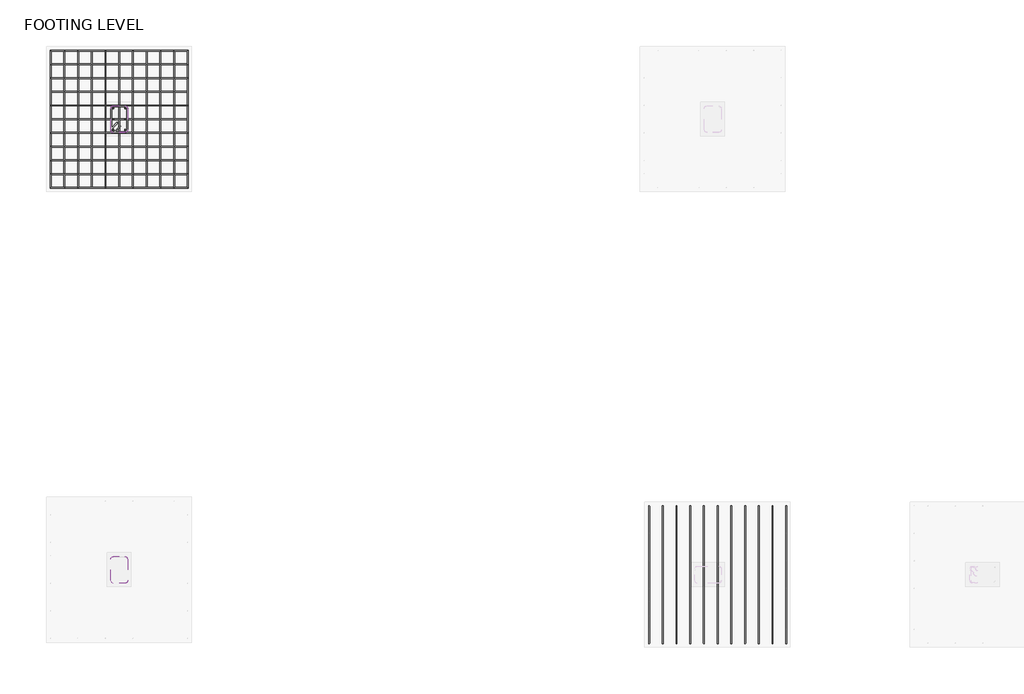
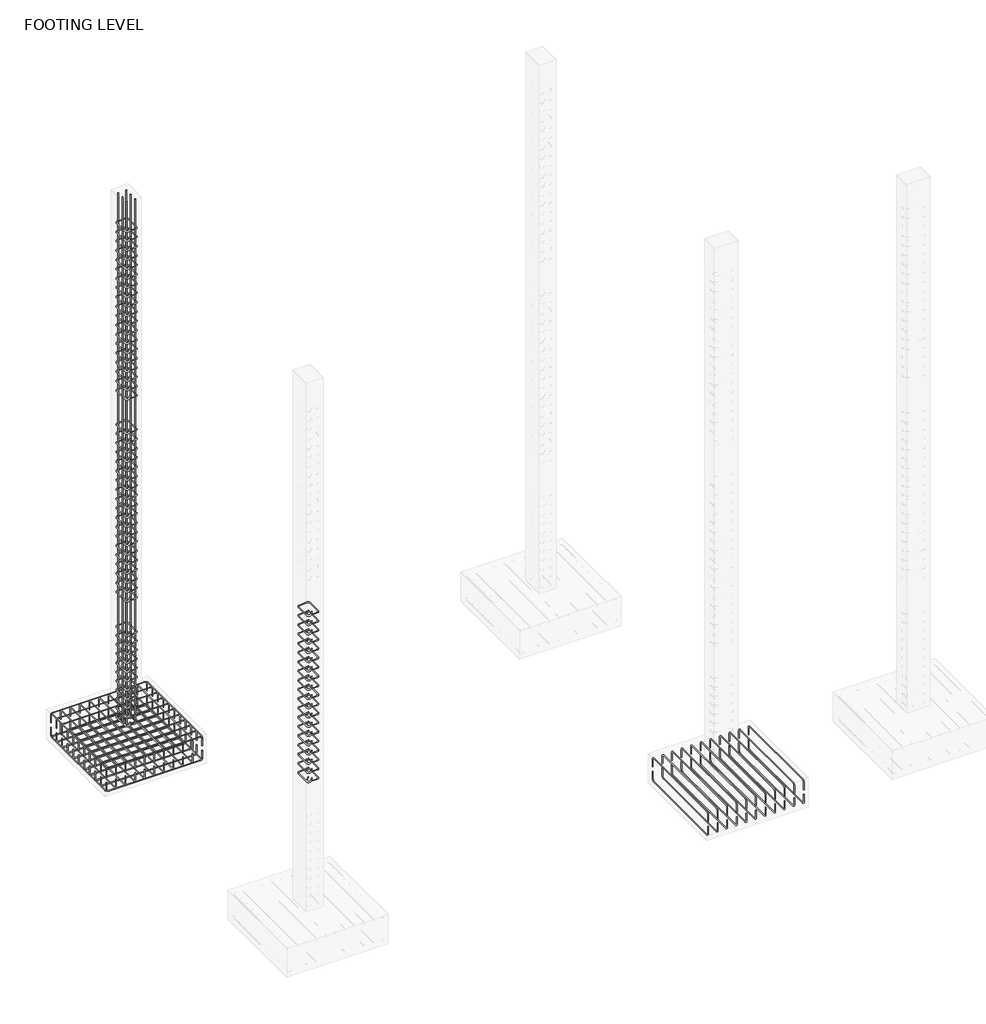
# One storey, part 7 of 9: 16 reinforcing bars.
"""IFC4 building model written with IfcOpenShell, lengths in millimetres."""

from ifc_helpers import new_model, si_unit, point, frame, origin, place, context, project, spatial, polyline, circle_curve, trimmed, segment, composite_curve, source, transform, mapped, element, save
from ifc_brep_helpers import swept_disk

model = new_model("IFC4")

# Units and contexts
model_context = context("Model", 3, world=origin())
ifc_project = project(units=[si_unit("LENGTHUNIT", "METRE", prefix="MILLI")], contexts=[model_context])

# Site, building, storey
site = spatial("IfcSite", under=ifc_project)
building = spatial("IfcBuilding", under=site)
storey = spatial("IfcBuildingStorey", under=building, Name="FOOTING LEVEL", Elevation=-1981.2)

# Reinforcing bars
placement = place(None, origin())
reinforcing_bar_shape = source(origin(), model_context, "Body", "SolidModel", [
    swept_disk(composite_curve([segment(polyline([(-5369.1458659, 8895.7158402, -2171.7), (-5369.1458659, 8895.7158402, -2057.4)]), True, "CONTINUOUS"), segment(trimmed(circle_curve(frame((-5369.1458659, 8862.3783402, -2057.4), z_axis=(1.0, 0.0, 0.0), x_axis=(0.0, 33.337499999999636, 0.0)), 33.3375), [point((-5369.1458659, 8895.7158402, -2057.4))], [point((-5369.1458659, 8862.3783402, -2024.0625))], True, "CARTESIAN"), True, "CONTINUOUS"), segment(polyline([(-5369.1458659, 8862.3783402, -2024.0625), (-5369.1458659, 7490.7783402, -2024.0625)]), True, "CONTINUOUS"), segment(trimmed(circle_curve(frame((-5369.1458659, 7490.7783402, -2057.4), z_axis=(1.0, 0.0, 0.0), x_axis=(0.0, 0.0, 33.33750000000009)), 33.3375), [point((-5369.1458659, 7490.7783402, -2024.0625))], [point((-5369.1458659, 7457.4408402, -2057.4))], True, "CARTESIAN"), True, "CONTINUOUS"), segment(polyline([(-5369.1458659, 7457.4408402, -2057.4), (-5369.1458659, 7457.4408402, -2171.7)]), True, "CONTINUOUS")], self_intersect=False), 4.7625),
])
element("IfcReinforcingBar", 1, at=placement, inside=storey, context=model_context, shape_type="MappedRepresentation", body=[
    mapped(reinforcing_bar_shape, transform((0.0, 0.0, 0.0), x_axis=(1.0, 0.0, 0.0), y_axis=(0.0, 1.0, 0.0), z_axis=(0.0, 0.0, 1.0))),
    mapped(reinforcing_bar_shape, transform((-143.8275, 0.0, 0.0), x_axis=(1.0, 0.0, 0.0), y_axis=(0.0, 1.0, 0.0), z_axis=(0.0, 0.0, 1.0))),
    mapped(reinforcing_bar_shape, transform((-287.655, 0.0, 0.0), x_axis=(1.0, 0.0, 0.0), y_axis=(0.0, 1.0, 0.0), z_axis=(0.0, 0.0, 1.0))),
    mapped(reinforcing_bar_shape, transform((-431.4825, 0.0, 0.0), x_axis=(1.0, 0.0, 0.0), y_axis=(0.0, 1.0, 0.0), z_axis=(0.0, 0.0, 1.0))),
    mapped(reinforcing_bar_shape, transform((-575.31, 0.0, 0.0), x_axis=(1.0, 0.0, 0.0), y_axis=(0.0, 1.0, 0.0), z_axis=(0.0, 0.0, 1.0))),
    mapped(reinforcing_bar_shape, transform((-719.1375, 0.0, 0.0), x_axis=(1.0, 0.0, 0.0), y_axis=(0.0, 1.0, 0.0), z_axis=(0.0, 0.0, 1.0))),
    mapped(reinforcing_bar_shape, transform((-862.965, 0.0, 0.0), x_axis=(1.0, 0.0, 0.0), y_axis=(0.0, 1.0, 0.0), z_axis=(0.0, 0.0, 1.0))),
    mapped(reinforcing_bar_shape, transform((-1006.7925, 0.0, 0.0), x_axis=(1.0, 0.0, 0.0), y_axis=(0.0, 1.0, 0.0), z_axis=(0.0, 0.0, 1.0))),
    mapped(reinforcing_bar_shape, transform((-1150.62, 0.0, 0.0), x_axis=(1.0, 0.0, 0.0), y_axis=(0.0, 1.0, 0.0), z_axis=(0.0, 0.0, 1.0))),
    mapped(reinforcing_bar_shape, transform((-1294.4475, 0.0, 0.0), x_axis=(1.0, 0.0, 0.0), y_axis=(0.0, 1.0, 0.0), z_axis=(0.0, 0.0, 1.0))),
    mapped(reinforcing_bar_shape, transform((-1438.275, 0.0, 0.0), x_axis=(1.0, 0.0, 0.0), y_axis=(0.0, 1.0, 0.0), z_axis=(0.0, 0.0, 1.0))),
])
reinforcing_bar_2_shape = source(origin(), model_context, "Body", "SolidModel", [
    swept_disk(composite_curve([segment(polyline([(-5369.1458659, 7457.4408402, -2247.9), (-5369.1458659, 7457.4408402, -2362.2)]), True, "CONTINUOUS"), segment(trimmed(circle_curve(frame((-5369.1458659, 7490.7783402, -2362.2), z_axis=(1.0, 0.0, 0.0), x_axis=(0.0, -33.337499999999636, 0.0)), 33.3375), [point((-5369.1458659, 7457.4408402, -2362.2))], [point((-5369.1458659, 7490.7783402, -2395.5375))], True, "CARTESIAN"), True, "CONTINUOUS"), segment(polyline([(-5369.1458659, 7490.7783402, -2395.5375), (-5369.1458659, 8862.3783402, -2395.5375)]), True, "CONTINUOUS"), segment(trimmed(circle_curve(frame((-5369.1458659, 8862.3783402, -2362.2), z_axis=(1.0, 0.0, 0.0), x_axis=(0.0, 0.0, -33.33750000000009)), 33.3375), [point((-5369.1458659, 8862.3783402, -2395.5375))], [point((-5369.1458659, 8895.7158402, -2362.2))], True, "CARTESIAN"), True, "CONTINUOUS"), segment(polyline([(-5369.1458659, 8895.7158402, -2362.2), (-5369.1458659, 8895.7158402, -2247.9)]), True, "CONTINUOUS")], self_intersect=False), 4.7625),
])
element("IfcReinforcingBar", 2, at=placement, inside=storey, context=model_context, shape_type="MappedRepresentation", body=[
    mapped(reinforcing_bar_2_shape, transform((0.0, 0.0, 0.0), x_axis=(1.0, 0.0, 0.0), y_axis=(0.0, 1.0, 0.0), z_axis=(0.0, 0.0, 1.0))),
    mapped(reinforcing_bar_2_shape, transform((-143.8275, 0.0, 0.0), x_axis=(1.0, 0.0, 0.0), y_axis=(0.0, 1.0, 0.0), z_axis=(0.0, 0.0, 1.0))),
    mapped(reinforcing_bar_2_shape, transform((-287.655, 0.0, 0.0), x_axis=(1.0, 0.0, 0.0), y_axis=(0.0, 1.0, 0.0), z_axis=(0.0, 0.0, 1.0))),
    mapped(reinforcing_bar_2_shape, transform((-431.4825, 0.0, 0.0), x_axis=(1.0, 0.0, 0.0), y_axis=(0.0, 1.0, 0.0), z_axis=(0.0, 0.0, 1.0))),
    mapped(reinforcing_bar_2_shape, transform((-575.31, 0.0, 0.0), x_axis=(1.0, 0.0, 0.0), y_axis=(0.0, 1.0, 0.0), z_axis=(0.0, 0.0, 1.0))),
    mapped(reinforcing_bar_2_shape, transform((-719.1375, 0.0, 0.0), x_axis=(1.0, 0.0, 0.0), y_axis=(0.0, 1.0, 0.0), z_axis=(0.0, 0.0, 1.0))),
    mapped(reinforcing_bar_2_shape, transform((-862.965, 0.0, 0.0), x_axis=(1.0, 0.0, 0.0), y_axis=(0.0, 1.0, 0.0), z_axis=(0.0, 0.0, 1.0))),
    mapped(reinforcing_bar_2_shape, transform((-1006.7925, 0.0, 0.0), x_axis=(1.0, 0.0, 0.0), y_axis=(0.0, 1.0, 0.0), z_axis=(0.0, 0.0, 1.0))),
    mapped(reinforcing_bar_2_shape, transform((-1150.62, 0.0, 0.0), x_axis=(1.0, 0.0, 0.0), y_axis=(0.0, 1.0, 0.0), z_axis=(0.0, 0.0, 1.0))),
    mapped(reinforcing_bar_2_shape, transform((-1294.4475, 0.0, 0.0), x_axis=(1.0, 0.0, 0.0), y_axis=(0.0, 1.0, 0.0), z_axis=(0.0, 0.0, 1.0))),
    mapped(reinforcing_bar_2_shape, transform((-1438.275, 0.0, 0.0), x_axis=(1.0, 0.0, 0.0), y_axis=(0.0, 1.0, 0.0), z_axis=(0.0, 0.0, 1.0))),
])
reinforcing_bar_3_shape = source(origin(), model_context, "Body", "SolidModel", [
    swept_disk(composite_curve([segment(polyline([(-11642.9458659, 13670.9158402, -2171.7), (-11642.9458659, 13670.9158402, -2057.4)]), True, "CONTINUOUS"), segment(trimmed(circle_curve(frame((-11642.9458659, 13637.5783402, -2057.4), z_axis=(1.0, 0.0, 0.0), x_axis=(0.0, 33.337499999999636, 0.0)), 33.3375), [point((-11642.9458659, 13670.9158402, -2057.4))], [point((-11642.9458659, 13637.5783402, -2024.0625))], True, "CARTESIAN"), True, "CONTINUOUS"), segment(polyline([(-11642.9458659, 13637.5783402, -2024.0625), (-11642.9458659, 12265.9783402, -2024.0625)]), True, "CONTINUOUS"), segment(trimmed(circle_curve(frame((-11642.9458659, 12265.9783402, -2057.4), z_axis=(1.0, 0.0, 0.0), x_axis=(0.0, 0.0, 33.33750000000009)), 33.3375), [point((-11642.9458659, 12265.9783402, -2024.0625))], [point((-11642.9458659, 12232.6408402, -2057.4))], True, "CARTESIAN"), True, "CONTINUOUS"), segment(polyline([(-11642.9458659, 12232.6408402, -2057.4), (-11642.9458659, 12232.6408402, -2171.7)]), True, "CONTINUOUS")], self_intersect=False), 4.7625),
])
element("IfcReinforcingBar", 3, at=placement, inside=storey, context=model_context, shape_type="MappedRepresentation", body=[
    mapped(reinforcing_bar_3_shape, transform((0.0, 0.0, 0.0), x_axis=(1.0, 0.0, 0.0), y_axis=(0.0, 1.0, 0.0), z_axis=(0.0, 0.0, 1.0))),
    mapped(reinforcing_bar_3_shape, transform((-143.8275, 0.0, 0.0), x_axis=(1.0, 0.0, 0.0), y_axis=(0.0, 1.0, 0.0), z_axis=(0.0, 0.0, 1.0))),
    mapped(reinforcing_bar_3_shape, transform((-287.655, 0.0, 0.0), x_axis=(1.0, 0.0, 0.0), y_axis=(0.0, 1.0, 0.0), z_axis=(0.0, 0.0, 1.0))),
    mapped(reinforcing_bar_3_shape, transform((-431.4825, 0.0, 0.0), x_axis=(1.0, 0.0, 0.0), y_axis=(0.0, 1.0, 0.0), z_axis=(0.0, 0.0, 1.0))),
    mapped(reinforcing_bar_3_shape, transform((-575.31, 0.0, 0.0), x_axis=(1.0, 0.0, 0.0), y_axis=(0.0, 1.0, 0.0), z_axis=(0.0, 0.0, 1.0))),
    mapped(reinforcing_bar_3_shape, transform((-719.1375, 0.0, 0.0), x_axis=(1.0, 0.0, 0.0), y_axis=(0.0, 1.0, 0.0), z_axis=(0.0, 0.0, 1.0))),
    mapped(reinforcing_bar_3_shape, transform((-862.965, 0.0, 0.0), x_axis=(1.0, 0.0, 0.0), y_axis=(0.0, 1.0, 0.0), z_axis=(0.0, 0.0, 1.0))),
    mapped(reinforcing_bar_3_shape, transform((-1006.7925, 0.0, 0.0), x_axis=(1.0, 0.0, 0.0), y_axis=(0.0, 1.0, 0.0), z_axis=(0.0, 0.0, 1.0))),
    mapped(reinforcing_bar_3_shape, transform((-1150.62, 0.0, 0.0), x_axis=(1.0, 0.0, 0.0), y_axis=(0.0, 1.0, 0.0), z_axis=(0.0, 0.0, 1.0))),
    mapped(reinforcing_bar_3_shape, transform((-1294.4475, 0.0, 0.0), x_axis=(1.0, 0.0, 0.0), y_axis=(0.0, 1.0, 0.0), z_axis=(0.0, 0.0, 1.0))),
    mapped(reinforcing_bar_3_shape, transform((-1438.275, 0.0, 0.0), x_axis=(1.0, 0.0, 0.0), y_axis=(0.0, 1.0, 0.0), z_axis=(0.0, 0.0, 1.0))),
])
reinforcing_bar_4_shape = source(origin(), model_context, "Body", "SolidModel", [
    swept_disk(composite_curve([segment(polyline([(-11642.9458659, 12232.6408402, -2247.9), (-11642.9458659, 12232.6408402, -2362.2)]), True, "CONTINUOUS"), segment(trimmed(circle_curve(frame((-11642.9458659, 12265.9783402, -2362.2), z_axis=(1.0, 0.0, 0.0), x_axis=(0.0, -33.337499999999636, 0.0)), 33.3375), [point((-11642.9458659, 12232.6408402, -2362.2))], [point((-11642.9458659, 12265.9783402, -2395.5375))], True, "CARTESIAN"), True, "CONTINUOUS"), segment(polyline([(-11642.9458659, 12265.9783402, -2395.5375), (-11642.9458659, 13637.5783402, -2395.5375)]), True, "CONTINUOUS"), segment(trimmed(circle_curve(frame((-11642.9458659, 13637.5783402, -2362.2), z_axis=(1.0, 0.0, 0.0), x_axis=(0.0, 0.0, -33.33750000000009)), 33.3375), [point((-11642.9458659, 13637.5783402, -2395.5375))], [point((-11642.9458659, 13670.9158402, -2362.2))], True, "CARTESIAN"), True, "CONTINUOUS"), segment(polyline([(-11642.9458659, 13670.9158402, -2362.2), (-11642.9458659, 13670.9158402, -2247.9)]), True, "CONTINUOUS")], self_intersect=False), 4.7625),
])
element("IfcReinforcingBar", 4, at=placement, inside=storey, context=model_context, shape_type="MappedRepresentation", body=[
    mapped(reinforcing_bar_4_shape, transform((0.0, 0.0, 0.0), x_axis=(1.0, 0.0, 0.0), y_axis=(0.0, 1.0, 0.0), z_axis=(0.0, 0.0, 1.0))),
    mapped(reinforcing_bar_4_shape, transform((-143.8275, 0.0, 0.0), x_axis=(1.0, 0.0, 0.0), y_axis=(0.0, 1.0, 0.0), z_axis=(0.0, 0.0, 1.0))),
    mapped(reinforcing_bar_4_shape, transform((-287.655, 0.0, 0.0), x_axis=(1.0, 0.0, 0.0), y_axis=(0.0, 1.0, 0.0), z_axis=(0.0, 0.0, 1.0))),
    mapped(reinforcing_bar_4_shape, transform((-431.4825, 0.0, 0.0), x_axis=(1.0, 0.0, 0.0), y_axis=(0.0, 1.0, 0.0), z_axis=(0.0, 0.0, 1.0))),
    mapped(reinforcing_bar_4_shape, transform((-575.31, 0.0, 0.0), x_axis=(1.0, 0.0, 0.0), y_axis=(0.0, 1.0, 0.0), z_axis=(0.0, 0.0, 1.0))),
    mapped(reinforcing_bar_4_shape, transform((-719.1375, 0.0, 0.0), x_axis=(1.0, 0.0, 0.0), y_axis=(0.0, 1.0, 0.0), z_axis=(0.0, 0.0, 1.0))),
    mapped(reinforcing_bar_4_shape, transform((-862.965, 0.0, 0.0), x_axis=(1.0, 0.0, 0.0), y_axis=(0.0, 1.0, 0.0), z_axis=(0.0, 0.0, 1.0))),
    mapped(reinforcing_bar_4_shape, transform((-1006.7925, 0.0, 0.0), x_axis=(1.0, 0.0, 0.0), y_axis=(0.0, 1.0, 0.0), z_axis=(0.0, 0.0, 1.0))),
    mapped(reinforcing_bar_4_shape, transform((-1150.62, 0.0, 0.0), x_axis=(1.0, 0.0, 0.0), y_axis=(0.0, 1.0, 0.0), z_axis=(0.0, 0.0, 1.0))),
    mapped(reinforcing_bar_4_shape, transform((-1294.4475, 0.0, 0.0), x_axis=(1.0, 0.0, 0.0), y_axis=(0.0, 1.0, 0.0), z_axis=(0.0, 0.0, 1.0))),
    mapped(reinforcing_bar_4_shape, transform((-1438.275, 0.0, 0.0), x_axis=(1.0, 0.0, 0.0), y_axis=(0.0, 1.0, 0.0), z_axis=(0.0, 0.0, 1.0))),
])
reinforcing_bar_5_shape = source(origin(), model_context, "Body", "SolidModel", [
    swept_disk(composite_curve([segment(polyline([(-13081.2208659, 13670.9158402, -2171.7), (-13081.2208659, 13670.9158402, -2057.4)]), True, "CONTINUOUS"), segment(trimmed(circle_curve(frame((-13047.8833659, 13670.9158402, -2057.4), z_axis=(0.0, 1.0, 0.0), x_axis=(-33.337500000001455, 0.0, 0.0)), 33.3375), [point((-13081.2208659, 13670.9158402, -2057.4))], [point((-13047.8833659, 13670.9158402, -2024.0625))], True, "CARTESIAN"), True, "CONTINUOUS"), segment(polyline([(-13047.8833659, 13670.9158402, -2024.0625), (-11676.2833659, 13670.9158402, -2024.0625)]), True, "CONTINUOUS"), segment(trimmed(circle_curve(frame((-11676.2833659, 13670.9158402, -2057.4), z_axis=(0.0, 1.0, 0.0), x_axis=(0.0, 0.0, 33.33750000000009)), 33.3375), [point((-11676.2833659, 13670.9158402, -2024.0625))], [point((-11642.9458659, 13670.9158402, -2057.4))], True, "CARTESIAN"), True, "CONTINUOUS"), segment(polyline([(-11642.9458659, 13670.9158402, -2057.4), (-11642.9458659, 13670.9158402, -2171.7)]), True, "CONTINUOUS")], self_intersect=False), 4.7625),
])
element("IfcReinforcingBar", 5, at=placement, inside=storey, context=model_context, shape_type="MappedRepresentation", body=[
    mapped(reinforcing_bar_5_shape, transform((0.0, 0.0, 0.0), x_axis=(1.0, 0.0, 0.0), y_axis=(0.0, 1.0, 0.0), z_axis=(0.0, 0.0, 1.0))),
    mapped(reinforcing_bar_5_shape, transform((0.0, -143.8275, 0.0), x_axis=(1.0, 0.0, 0.0), y_axis=(0.0, 1.0, 0.0), z_axis=(0.0, 0.0, 1.0))),
    mapped(reinforcing_bar_5_shape, transform((0.0, -287.655, 0.0), x_axis=(1.0, 0.0, 0.0), y_axis=(0.0, 1.0, 0.0), z_axis=(0.0, 0.0, 1.0))),
    mapped(reinforcing_bar_5_shape, transform((0.0, -431.4825, 0.0), x_axis=(1.0, 0.0, 0.0), y_axis=(0.0, 1.0, 0.0), z_axis=(0.0, 0.0, 1.0))),
    mapped(reinforcing_bar_5_shape, transform((0.0, -575.31, 0.0), x_axis=(1.0, 0.0, 0.0), y_axis=(0.0, 1.0, 0.0), z_axis=(0.0, 0.0, 1.0))),
    mapped(reinforcing_bar_5_shape, transform((0.0, -719.1375, 0.0), x_axis=(1.0, 0.0, 0.0), y_axis=(0.0, 1.0, 0.0), z_axis=(0.0, 0.0, 1.0))),
    mapped(reinforcing_bar_5_shape, transform((0.0, -862.965, 0.0), x_axis=(1.0, 0.0, 0.0), y_axis=(0.0, 1.0, 0.0), z_axis=(0.0, 0.0, 1.0))),
    mapped(reinforcing_bar_5_shape, transform((0.0, -1006.7925, 0.0), x_axis=(1.0, 0.0, 0.0), y_axis=(0.0, 1.0, 0.0), z_axis=(0.0, 0.0, 1.0))),
    mapped(reinforcing_bar_5_shape, transform((0.0, -1150.62, 0.0), x_axis=(1.0, 0.0, 0.0), y_axis=(0.0, 1.0, 0.0), z_axis=(0.0, 0.0, 1.0))),
    mapped(reinforcing_bar_5_shape, transform((0.0, -1294.4475, 0.0), x_axis=(1.0, 0.0, 0.0), y_axis=(0.0, 1.0, 0.0), z_axis=(0.0, 0.0, 1.0))),
    mapped(reinforcing_bar_5_shape, transform((0.0, -1438.275, 0.0), x_axis=(1.0, 0.0, 0.0), y_axis=(0.0, 1.0, 0.0), z_axis=(0.0, 0.0, 1.0))),
])
reinforcing_bar_6_shape = source(origin(), model_context, "Body", "SolidModel", [
    swept_disk(composite_curve([segment(polyline([(-13081.2208659, 12232.6408402, -2247.9), (-13081.2208659, 12232.6408402, -2362.2)]), True, "CONTINUOUS"), segment(trimmed(circle_curve(frame((-13047.8833659, 12232.6408402, -2362.2), z_axis=(0.0, -1.0, 0.0), x_axis=(-33.337500000001455, 0.0, 0.0)), 33.3375), [point((-13081.2208659, 12232.6408402, -2362.2))], [point((-13047.8833659, 12232.6408402, -2395.5375))], True, "CARTESIAN"), True, "CONTINUOUS"), segment(polyline([(-13047.8833659, 12232.6408402, -2395.5375), (-11676.2833659, 12232.6408402, -2395.5375)]), True, "CONTINUOUS"), segment(trimmed(circle_curve(frame((-11676.2833659, 12232.6408402, -2362.2), z_axis=(0.0, -1.0, 0.0), x_axis=(0.0, 0.0, -33.33750000000009)), 33.3375), [point((-11676.2833659, 12232.6408402, -2395.5375))], [point((-11642.9458659, 12232.6408402, -2362.2))], True, "CARTESIAN"), True, "CONTINUOUS"), segment(polyline([(-11642.9458659, 12232.6408402, -2362.2), (-11642.9458659, 12232.6408402, -2247.9)]), True, "CONTINUOUS")], self_intersect=False), 4.7625),
])
element("IfcReinforcingBar", 6, at=placement, inside=storey, context=model_context, shape_type="MappedRepresentation", body=[
    mapped(reinforcing_bar_6_shape, transform((0.0, 0.0, 0.0), x_axis=(1.0, 0.0, 0.0), y_axis=(0.0, 1.0, 0.0), z_axis=(0.0, 0.0, 1.0))),
    mapped(reinforcing_bar_6_shape, transform((0.0, 143.8275, 0.0), x_axis=(1.0, 0.0, 0.0), y_axis=(0.0, 1.0, 0.0), z_axis=(0.0, 0.0, 1.0))),
    mapped(reinforcing_bar_6_shape, transform((0.0, 287.655, 0.0), x_axis=(1.0, 0.0, 0.0), y_axis=(0.0, 1.0, 0.0), z_axis=(0.0, 0.0, 1.0))),
    mapped(reinforcing_bar_6_shape, transform((0.0, 431.4825, 0.0), x_axis=(1.0, 0.0, 0.0), y_axis=(0.0, 1.0, 0.0), z_axis=(0.0, 0.0, 1.0))),
    mapped(reinforcing_bar_6_shape, transform((0.0, 575.31, 0.0), x_axis=(1.0, 0.0, 0.0), y_axis=(0.0, 1.0, 0.0), z_axis=(0.0, 0.0, 1.0))),
    mapped(reinforcing_bar_6_shape, transform((0.0, 719.1375, 0.0), x_axis=(1.0, 0.0, 0.0), y_axis=(0.0, 1.0, 0.0), z_axis=(0.0, 0.0, 1.0))),
    mapped(reinforcing_bar_6_shape, transform((0.0, 862.965, 0.0), x_axis=(1.0, 0.0, 0.0), y_axis=(0.0, 1.0, 0.0), z_axis=(0.0, 0.0, 1.0))),
    mapped(reinforcing_bar_6_shape, transform((0.0, 1006.7925, 0.0), x_axis=(1.0, 0.0, 0.0), y_axis=(0.0, 1.0, 0.0), z_axis=(0.0, 0.0, 1.0))),
    mapped(reinforcing_bar_6_shape, transform((0.0, 1150.62, 0.0), x_axis=(1.0, 0.0, 0.0), y_axis=(0.0, 1.0, 0.0), z_axis=(0.0, 0.0, 1.0))),
    mapped(reinforcing_bar_6_shape, transform((0.0, 1294.4475, 0.0), x_axis=(1.0, 0.0, 0.0), y_axis=(0.0, 1.0, 0.0), z_axis=(0.0, 0.0, 1.0))),
    mapped(reinforcing_bar_6_shape, transform((0.0, 1438.275, 0.0), x_axis=(1.0, 0.0, 0.0), y_axis=(0.0, 1.0, 0.0), z_axis=(0.0, 0.0, 1.0))),
])
reinforcing_bar_7_shape = source(origin(), model_context, "Body", "SolidModel", [
    swept_disk(composite_curve([segment(polyline([(-12382.3821491, 12914.3555175, -1938.3375), (-12439.2463461, 12857.4913204, -1938.3375)]), True, "CONTINUOUS"), segment(trimmed(circle_curve(frame((-12422.4083659, 12840.6533402, -1938.3375), z_axis=(0.0, 0.0, 1.0), x_axis=(-16.837980199999947, 16.837980199999947, 0.0)), 23.8125), [point((-12439.2463461, 12857.4913204, -1938.3375))], [point((-12422.4083659, 12816.8408402, -1938.3375))], True, "CARTESIAN"), True, "CONTINUOUS"), segment(polyline([(-12422.4083659, 12816.8408402, -1938.3375), (-12301.7583659, 12816.8408402, -1938.3375)]), True, "CONTINUOUS"), segment(trimmed(circle_curve(frame((-12301.7583659, 12840.6533402, -1938.3375), z_axis=(0.0, 0.0, 1.0), x_axis=(0.0, -23.8125, 0.0)), 23.8125), [point((-12301.7583659, 12816.8408402, -1938.3375))], [point((-12277.9458659, 12840.6533402, -1938.3375))], True, "CARTESIAN"), True, "CONTINUOUS"), segment(polyline([(-12277.9458659, 12840.6533402, -1938.3375), (-12277.9458659, 13062.9033402, -1938.3375)]), True, "CONTINUOUS"), segment(trimmed(circle_curve(frame((-12301.7203098, 13062.9033402, -1939.6832232), z_axis=(-0.056513312022656255, 0.0, 0.9984018457335854), x_axis=(23.774443900001643, 0.0, 1.3457231999998385)), 23.8125), [point((-12277.9458659, 13062.9033402, -1938.3375))], [point((-12301.7203098, 13086.7158402, -1939.6832232))], True, "CARTESIAN"), True, "CONTINUOUS"), segment(polyline([(-12301.7203098, 13086.7158402, -1939.6832232), (-12422.4464219, 13086.7158402, -1946.5167768)]), True, "CONTINUOUS"), segment(trimmed(circle_curve(frame((-12422.4464219, 13062.9033402, -1946.5167768), z_axis=(-0.056513312022656255, 0.0, 0.9984018457335854), x_axis=(0.0, 23.8125, 0.0)), 23.8125), [point((-12422.4464219, 13086.7158402, -1946.5167768))], [point((-12446.2208659, 13062.9033402, -1947.8625))], True, "CARTESIAN"), True, "CONTINUOUS"), segment(polyline([(-12446.2208659, 13062.9033402, -1947.8625), (-12446.2208659, 12840.6533402, -1947.8625)]), True, "CONTINUOUS"), segment(trimmed(circle_curve(frame((-12422.4083659, 12840.6533402, -1947.8625), z_axis=(0.0, 0.0, 1.0), x_axis=(-23.8125, 0.0, 0.0)), 23.8125), [point((-12446.2208659, 12840.6533402, -1947.8625))], [point((-12405.5703857, 12823.81536, -1947.8625))], True, "CARTESIAN"), True, "CONTINUOUS"), segment(polyline([(-12405.5703857, 12823.81536, -1947.8625), (-12348.7061886, 12880.679557, -1947.8625)]), True, "CONTINUOUS")], self_intersect=False), 4.7625),
])
element("IfcReinforcingBar", 7, at=placement, inside=storey, context=model_context, shape_type="MappedRepresentation", body=[
    mapped(reinforcing_bar_7_shape, transform((0.0, 0.0, 0.0), x_axis=(1.0, 0.0, 0.0), y_axis=(0.0, 1.0, 0.0), z_axis=(0.0, 0.0, 1.0))),
    mapped(reinforcing_bar_7_shape, transform((0.0, 0.0, 143.3979062), x_axis=(1.0, 0.0, 0.0), y_axis=(0.0, 1.0, 0.0), z_axis=(0.0, 0.0, 1.0))),
    mapped(reinforcing_bar_7_shape, transform((0.0, 0.0, 286.7958125), x_axis=(1.0, 0.0, 0.0), y_axis=(0.0, 1.0, 0.0), z_axis=(0.0, 0.0, 1.0))),
    mapped(reinforcing_bar_7_shape, transform((0.0, 0.0, 430.1937187), x_axis=(1.0, 0.0, 0.0), y_axis=(0.0, 1.0, 0.0), z_axis=(0.0, 0.0, 1.0))),
    mapped(reinforcing_bar_7_shape, transform((0.0, 0.0, 573.5916249), x_axis=(1.0, 0.0, 0.0), y_axis=(0.0, 1.0, 0.0), z_axis=(0.0, 0.0, 1.0))),
    mapped(reinforcing_bar_7_shape, transform((0.0, 0.0, 716.9895311), x_axis=(1.0, 0.0, 0.0), y_axis=(0.0, 1.0, 0.0), z_axis=(0.0, 0.0, 1.0))),
    mapped(reinforcing_bar_7_shape, transform((0.0, 0.0, 860.3874374), x_axis=(1.0, 0.0, 0.0), y_axis=(0.0, 1.0, 0.0), z_axis=(0.0, 0.0, 1.0))),
    mapped(reinforcing_bar_7_shape, transform((0.0, 0.0, 1003.7853436), x_axis=(1.0, 0.0, 0.0), y_axis=(0.0, 1.0, 0.0), z_axis=(0.0, 0.0, 1.0))),
    mapped(reinforcing_bar_7_shape, transform((0.0, 0.0, 1147.1832498), x_axis=(1.0, 0.0, 0.0), y_axis=(0.0, 1.0, 0.0), z_axis=(0.0, 0.0, 1.0))),
    mapped(reinforcing_bar_7_shape, transform((0.0, 0.0, 1290.581156), x_axis=(1.0, 0.0, 0.0), y_axis=(0.0, 1.0, 0.0), z_axis=(0.0, 0.0, 1.0))),
    mapped(reinforcing_bar_7_shape, transform((0.0, 0.0, 1433.9790623), x_axis=(1.0, 0.0, 0.0), y_axis=(0.0, 1.0, 0.0), z_axis=(0.0, 0.0, 1.0))),
])
element("IfcReinforcingBar", 8, at=placement, inside=storey, context=model_context, shape_type="SolidModel", body=[
    swept_disk(composite_curve([segment(polyline([(-12423.8882737, 13065.2596793, -1943.1), (-12423.8882737, 13065.2596793, 6362.7)]), True, "CONTINUOUS")], self_intersect=False), 6.35),
])
element("IfcReinforcingBar", 9, at=placement, inside=storey, context=model_context, shape_type="SolidModel", body=[
    swept_disk(composite_curve([segment(polyline([(-12300.2784581, 13065.2596793, -1943.1), (-12300.2784581, 13065.2596793, 6362.7)]), True, "CONTINUOUS")], self_intersect=False), 6.35),
])
element("IfcReinforcingBar", 10, at=placement, inside=storey, context=model_context, shape_type="SolidModel", body=[
    swept_disk(composite_curve([segment(polyline([(-12423.8882737, 12838.2970011, -1943.1), (-12423.8882737, 12838.2970011, 6362.7)]), True, "CONTINUOUS")], self_intersect=False), 6.35),
])
element("IfcReinforcingBar", 11, at=placement, inside=storey, context=model_context, shape_type="SolidModel", body=[
    swept_disk(composite_curve([segment(polyline([(-12300.2784581, 12838.2970011, -1943.1), (-12300.2784581, 12838.2970011, 6362.7)]), True, "CONTINUOUS")], self_intersect=False), 6.35),
])
element("IfcReinforcingBar", 12, at=placement, inside=storey, context=model_context, shape_type="SolidModel", body=[
    swept_disk(composite_curve([segment(polyline([(-12423.8882737, 12952.5970011, -1943.1), (-12423.8882737, 12952.5970011, 6362.7)]), True, "CONTINUOUS")], self_intersect=False), 6.35),
])
element("IfcReinforcingBar", 13, at=placement, inside=storey, context=model_context, shape_type="SolidModel", body=[
    swept_disk(composite_curve([segment(polyline([(-12300.2784581, 12952.5970011, -1943.1), (-12300.2784581, 12952.5970011, 6362.7)]), True, "CONTINUOUS")], self_intersect=False), 6.35),
])
reinforcing_bar_8_shape = source(origin(), model_context, "Body", "SolidModel", [
    swept_disk(composite_curve([segment(polyline([(-12382.3821491, 12914.3555175, 42.8625), (-12439.2463461, 12857.4913204, 42.8625)]), True, "CONTINUOUS"), segment(trimmed(circle_curve(frame((-12422.4083659, 12840.6533402, 42.8625), z_axis=(0.0, 0.0, 1.0), x_axis=(-16.837980199999947, 16.837980199999947, 0.0)), 23.8125), [point((-12439.2463461, 12857.4913204, 42.8625))], [point((-12422.4083659, 12816.8408402, 42.8625))], True, "CARTESIAN"), True, "CONTINUOUS"), segment(polyline([(-12422.4083659, 12816.8408402, 42.8625), (-12301.7583659, 12816.8408402, 42.8625)]), True, "CONTINUOUS"), segment(trimmed(circle_curve(frame((-12301.7583659, 12840.6533402, 42.8625), z_axis=(0.0, 0.0, 1.0), x_axis=(0.0, -23.8125, 0.0)), 23.8125), [point((-12301.7583659, 12816.8408402, 42.8625))], [point((-12277.9458659, 12840.6533402, 42.8625))], True, "CARTESIAN"), True, "CONTINUOUS"), segment(polyline([(-12277.9458659, 12840.6533402, 42.8625), (-12277.9458659, 13062.9033402, 42.8625)]), True, "CONTINUOUS"), segment(trimmed(circle_curve(frame((-12301.7203098, 13062.9033402, 41.5167768), z_axis=(-0.056513312022656255, 0.0, 0.9984018457335854), x_axis=(23.774443900001643, 0.0, 1.3457231999999948)), 23.8125), [point((-12277.9458659, 13062.9033402, 42.8625))], [point((-12301.7203098, 13086.7158402, 41.5167768))], True, "CARTESIAN"), True, "CONTINUOUS"), segment(polyline([(-12301.7203098, 13086.7158402, 41.5167768), (-12422.4464219, 13086.7158402, 34.6832232)]), True, "CONTINUOUS"), segment(trimmed(circle_curve(frame((-12422.4464219, 13062.9033402, 34.6832232), z_axis=(-0.056513312022656255, 0.0, 0.9984018457335854), x_axis=(0.0, 23.8125, 0.0)), 23.8125), [point((-12422.4464219, 13086.7158402, 34.6832232))], [point((-12446.2208659, 13062.9033402, 33.3375))], True, "CARTESIAN"), True, "CONTINUOUS"), segment(polyline([(-12446.2208659, 13062.9033402, 33.3375), (-12446.2208659, 12840.6533402, 33.3375)]), True, "CONTINUOUS"), segment(trimmed(circle_curve(frame((-12422.4083659, 12840.6533402, 33.3375), z_axis=(0.0, 0.0, 1.0), x_axis=(-23.8125, 0.0, 0.0)), 23.8125), [point((-12446.2208659, 12840.6533402, 33.3375))], [point((-12405.5703857, 12823.81536, 33.3375))], True, "CARTESIAN"), True, "CONTINUOUS"), segment(polyline([(-12405.5703857, 12823.81536, 33.3375), (-12348.7061886, 12880.679557, 33.3375)]), True, "CONTINUOUS")], self_intersect=False), 4.7625),
])
element("IfcReinforcingBar", 14, at=placement, inside=storey, context=model_context, shape_type="MappedRepresentation", body=[
    mapped(reinforcing_bar_8_shape, transform((0.0, 0.0, 0.0), x_axis=(1.0, 0.0, 0.0), y_axis=(0.0, 1.0, 0.0), z_axis=(0.0, 0.0, 1.0))),
    mapped(reinforcing_bar_8_shape, transform((0.0, 0.0, 147.8567446), x_axis=(1.0, 0.0, 0.0), y_axis=(0.0, 1.0, 0.0), z_axis=(0.0, 0.0, 1.0))),
    mapped(reinforcing_bar_8_shape, transform((0.0, 0.0, 295.7134892), x_axis=(1.0, 0.0, 0.0), y_axis=(0.0, 1.0, 0.0), z_axis=(0.0, 0.0, 1.0))),
    mapped(reinforcing_bar_8_shape, transform((0.0, 0.0, 443.5702338), x_axis=(1.0, 0.0, 0.0), y_axis=(0.0, 1.0, 0.0), z_axis=(0.0, 0.0, 1.0))),
    mapped(reinforcing_bar_8_shape, transform((0.0, 0.0, 591.4269784), x_axis=(1.0, 0.0, 0.0), y_axis=(0.0, 1.0, 0.0), z_axis=(0.0, 0.0, 1.0))),
    mapped(reinforcing_bar_8_shape, transform((0.0, 0.0, 739.283723), x_axis=(1.0, 0.0, 0.0), y_axis=(0.0, 1.0, 0.0), z_axis=(0.0, 0.0, 1.0))),
    mapped(reinforcing_bar_8_shape, transform((0.0, 0.0, 887.1404675), x_axis=(1.0, 0.0, 0.0), y_axis=(0.0, 1.0, 0.0), z_axis=(0.0, 0.0, 1.0))),
    mapped(reinforcing_bar_8_shape, transform((0.0, 0.0, 1034.9972121), x_axis=(1.0, 0.0, 0.0), y_axis=(0.0, 1.0, 0.0), z_axis=(0.0, 0.0, 1.0))),
    mapped(reinforcing_bar_8_shape, transform((0.0, 0.0, 1182.8539567), x_axis=(1.0, 0.0, 0.0), y_axis=(0.0, 1.0, 0.0), z_axis=(0.0, 0.0, 1.0))),
    mapped(reinforcing_bar_8_shape, transform((0.0, 0.0, 1330.7107013), x_axis=(1.0, 0.0, 0.0), y_axis=(0.0, 1.0, 0.0), z_axis=(0.0, 0.0, 1.0))),
    mapped(reinforcing_bar_8_shape, transform((0.0, 0.0, 1478.5674459), x_axis=(1.0, 0.0, 0.0), y_axis=(0.0, 1.0, 0.0), z_axis=(0.0, 0.0, 1.0))),
    mapped(reinforcing_bar_8_shape, transform((0.0, 0.0, 1626.4241905), x_axis=(1.0, 0.0, 0.0), y_axis=(0.0, 1.0, 0.0), z_axis=(0.0, 0.0, 1.0))),
    mapped(reinforcing_bar_8_shape, transform((0.0, 0.0, 1774.2809351), x_axis=(1.0, 0.0, 0.0), y_axis=(0.0, 1.0, 0.0), z_axis=(0.0, 0.0, 1.0))),
    mapped(reinforcing_bar_8_shape, transform((0.0, 0.0, 1922.1376797), x_axis=(1.0, 0.0, 0.0), y_axis=(0.0, 1.0, 0.0), z_axis=(0.0, 0.0, 1.0))),
    mapped(reinforcing_bar_8_shape, transform((0.0, 0.0, 2069.9944243), x_axis=(1.0, 0.0, 0.0), y_axis=(0.0, 1.0, 0.0), z_axis=(0.0, 0.0, 1.0))),
    mapped(reinforcing_bar_8_shape, transform((0.0, 0.0, 2217.8511689), x_axis=(1.0, 0.0, 0.0), y_axis=(0.0, 1.0, 0.0), z_axis=(0.0, 0.0, 1.0))),
    mapped(reinforcing_bar_8_shape, transform((0.0, 0.0, 2365.7079134), x_axis=(1.0, 0.0, 0.0), y_axis=(0.0, 1.0, 0.0), z_axis=(0.0, 0.0, 1.0))),
    mapped(reinforcing_bar_8_shape, transform((0.0, 0.0, 2513.564658), x_axis=(1.0, 0.0, 0.0), y_axis=(0.0, 1.0, 0.0), z_axis=(0.0, 0.0, 1.0))),
    mapped(reinforcing_bar_8_shape, transform((0.0, 0.0, 2661.4214026), x_axis=(1.0, 0.0, 0.0), y_axis=(0.0, 1.0, 0.0), z_axis=(0.0, 0.0, 1.0))),
])
reinforcing_bar_9_shape = source(origin(), model_context, "Body", "SolidModel", [
    swept_disk(composite_curve([segment(polyline([(-12382.3821491, 12914.3555175, 3243.2625), (-12439.2463461, 12857.4913204, 3243.2625)]), True, "CONTINUOUS"), segment(trimmed(circle_curve(frame((-12422.4083659, 12840.6533402, 3243.2625), z_axis=(0.0, 0.0, 1.0), x_axis=(-16.837980199999947, 16.837980199999947, 0.0)), 23.8125), [point((-12439.2463461, 12857.4913204, 3243.2625))], [point((-12422.4083659, 12816.8408402, 3243.2625))], True, "CARTESIAN"), True, "CONTINUOUS"), segment(polyline([(-12422.4083659, 12816.8408402, 3243.2625), (-12301.7583659, 12816.8408402, 3243.2625)]), True, "CONTINUOUS"), segment(trimmed(circle_curve(frame((-12301.7583659, 12840.6533402, 3243.2625), z_axis=(0.0, 0.0, 1.0), x_axis=(0.0, -23.8125, 0.0)), 23.8125), [point((-12301.7583659, 12816.8408402, 3243.2625))], [point((-12277.9458659, 12840.6533402, 3243.2625))], True, "CARTESIAN"), True, "CONTINUOUS"), segment(polyline([(-12277.9458659, 12840.6533402, 3243.2625), (-12277.9458659, 13062.9033402, 3243.2625)]), True, "CONTINUOUS"), segment(trimmed(circle_curve(frame((-12301.7203098, 13062.9033402, 3241.9167768), z_axis=(-0.056513312022656255, 0.0, 0.9984018457335854), x_axis=(23.774443900001643, 0.0, 1.345723199999611)), 23.8125), [point((-12277.9458659, 13062.9033402, 3243.2625))], [point((-12301.7203098, 13086.7158402, 3241.9167768))], True, "CARTESIAN"), True, "CONTINUOUS"), segment(polyline([(-12301.7203098, 13086.7158402, 3241.9167768), (-12422.4464219, 13086.7158402, 3235.0832232)]), True, "CONTINUOUS"), segment(trimmed(circle_curve(frame((-12422.4464219, 13062.9033402, 3235.0832232), z_axis=(-0.056513312022656255, 0.0, 0.9984018457335854), x_axis=(0.0, 23.8125, 0.0)), 23.8125), [point((-12422.4464219, 13086.7158402, 3235.0832232))], [point((-12446.2208659, 13062.9033402, 3233.7375))], True, "CARTESIAN"), True, "CONTINUOUS"), segment(polyline([(-12446.2208659, 13062.9033402, 3233.7375), (-12446.2208659, 12840.6533402, 3233.7375)]), True, "CONTINUOUS"), segment(trimmed(circle_curve(frame((-12422.4083659, 12840.6533402, 3233.7375), z_axis=(0.0, 0.0, 1.0), x_axis=(-23.8125, 0.0, 0.0)), 23.8125), [point((-12446.2208659, 12840.6533402, 3233.7375))], [point((-12405.5703857, 12823.81536, 3233.7375))], True, "CARTESIAN"), True, "CONTINUOUS"), segment(polyline([(-12405.5703857, 12823.81536, 3233.7375), (-12348.7061886, 12880.679557, 3233.7375)]), True, "CONTINUOUS")], self_intersect=False), 4.7625),
])
element("IfcReinforcingBar", 15, at=placement, inside=storey, context=model_context, shape_type="MappedRepresentation", body=[
    mapped(reinforcing_bar_9_shape, transform((0.0, 0.0, 0.0), x_axis=(1.0, 0.0, 0.0), y_axis=(0.0, 1.0, 0.0), z_axis=(0.0, 0.0, 1.0))),
    mapped(reinforcing_bar_9_shape, transform((0.0, 0.0, 147.8770493), x_axis=(1.0, 0.0, 0.0), y_axis=(0.0, 1.0, 0.0), z_axis=(0.0, 0.0, 1.0))),
    mapped(reinforcing_bar_9_shape, transform((0.0, 0.0, 295.7540986), x_axis=(1.0, 0.0, 0.0), y_axis=(0.0, 1.0, 0.0), z_axis=(0.0, 0.0, 1.0))),
    mapped(reinforcing_bar_9_shape, transform((0.0, 0.0, 443.6311479), x_axis=(1.0, 0.0, 0.0), y_axis=(0.0, 1.0, 0.0), z_axis=(0.0, 0.0, 1.0))),
    mapped(reinforcing_bar_9_shape, transform((0.0, 0.0, 591.5081972), x_axis=(1.0, 0.0, 0.0), y_axis=(0.0, 1.0, 0.0), z_axis=(0.0, 0.0, 1.0))),
    mapped(reinforcing_bar_9_shape, transform((0.0, 0.0, 739.3852464), x_axis=(1.0, 0.0, 0.0), y_axis=(0.0, 1.0, 0.0), z_axis=(0.0, 0.0, 1.0))),
    mapped(reinforcing_bar_9_shape, transform((0.0, 0.0, 887.2622957), x_axis=(1.0, 0.0, 0.0), y_axis=(0.0, 1.0, 0.0), z_axis=(0.0, 0.0, 1.0))),
    mapped(reinforcing_bar_9_shape, transform((0.0, 0.0, 1035.139345), x_axis=(1.0, 0.0, 0.0), y_axis=(0.0, 1.0, 0.0), z_axis=(0.0, 0.0, 1.0))),
    mapped(reinforcing_bar_9_shape, transform((0.0, 0.0, 1183.0163943), x_axis=(1.0, 0.0, 0.0), y_axis=(0.0, 1.0, 0.0), z_axis=(0.0, 0.0, 1.0))),
    mapped(reinforcing_bar_9_shape, transform((0.0, 0.0, 1330.8934436), x_axis=(1.0, 0.0, 0.0), y_axis=(0.0, 1.0, 0.0), z_axis=(0.0, 0.0, 1.0))),
    mapped(reinforcing_bar_9_shape, transform((0.0, 0.0, 1478.7704929), x_axis=(1.0, 0.0, 0.0), y_axis=(0.0, 1.0, 0.0), z_axis=(0.0, 0.0, 1.0))),
    mapped(reinforcing_bar_9_shape, transform((0.0, 0.0, 1626.6475422), x_axis=(1.0, 0.0, 0.0), y_axis=(0.0, 1.0, 0.0), z_axis=(0.0, 0.0, 1.0))),
    mapped(reinforcing_bar_9_shape, transform((0.0, 0.0, 1774.5245915), x_axis=(1.0, 0.0, 0.0), y_axis=(0.0, 1.0, 0.0), z_axis=(0.0, 0.0, 1.0))),
    mapped(reinforcing_bar_9_shape, transform((0.0, 0.0, 1922.4016408), x_axis=(1.0, 0.0, 0.0), y_axis=(0.0, 1.0, 0.0), z_axis=(0.0, 0.0, 1.0))),
    mapped(reinforcing_bar_9_shape, transform((0.0, 0.0, 2070.2786901), x_axis=(1.0, 0.0, 0.0), y_axis=(0.0, 1.0, 0.0), z_axis=(0.0, 0.0, 1.0))),
    mapped(reinforcing_bar_9_shape, transform((0.0, 0.0, 2218.1557393), x_axis=(1.0, 0.0, 0.0), y_axis=(0.0, 1.0, 0.0), z_axis=(0.0, 0.0, 1.0))),
    mapped(reinforcing_bar_9_shape, transform((0.0, 0.0, 2366.0327886), x_axis=(1.0, 0.0, 0.0), y_axis=(0.0, 1.0, 0.0), z_axis=(0.0, 0.0, 1.0))),
    mapped(reinforcing_bar_9_shape, transform((0.0, 0.0, 2513.9098379), x_axis=(1.0, 0.0, 0.0), y_axis=(0.0, 1.0, 0.0), z_axis=(0.0, 0.0, 1.0))),
    mapped(reinforcing_bar_9_shape, transform((0.0, 0.0, 2661.7868872), x_axis=(1.0, 0.0, 0.0), y_axis=(0.0, 1.0, 0.0), z_axis=(0.0, 0.0, 1.0))),
])
reinforcing_bar_10_shape = source(origin(), model_context, "Body", "SolidModel", [
    swept_disk(composite_curve([segment(polyline([(-12382.3821491, 8189.9555175, 42.8625), (-12439.2463461, 8133.0913204, 42.8625)]), True, "CONTINUOUS"), segment(trimmed(circle_curve(frame((-12422.4083659, 8116.2533402, 42.8625), z_axis=(0.0, 0.0, 1.0), x_axis=(-16.837980199999947, 16.837980199999947, 0.0)), 23.8125), [point((-12439.2463461, 8133.0913204, 42.8625))], [point((-12422.4083659, 8092.4408402, 42.8625))], True, "CARTESIAN"), True, "CONTINUOUS"), segment(polyline([(-12422.4083659, 8092.4408402, 42.8625), (-12301.7583659, 8092.4408402, 42.8625)]), True, "CONTINUOUS"), segment(trimmed(circle_curve(frame((-12301.7583659, 8116.2533402, 42.8625), z_axis=(0.0, 0.0, 1.0), x_axis=(0.0, -23.8125, 0.0)), 23.8125), [point((-12301.7583659, 8092.4408402, 42.8625))], [point((-12277.9458659, 8116.2533402, 42.8625))], True, "CARTESIAN"), True, "CONTINUOUS"), segment(polyline([(-12277.9458659, 8116.2533402, 42.8625), (-12277.9458659, 8338.5033402, 42.8625)]), True, "CONTINUOUS"), segment(trimmed(circle_curve(frame((-12301.7203098, 8338.5033402, 41.5167768), z_axis=(-0.056513312022656255, 0.0, 0.9984018457335854), x_axis=(23.774443900001643, 0.0, 1.3457231999999948)), 23.8125), [point((-12277.9458659, 8338.5033402, 42.8625))], [point((-12301.7203098, 8362.3158402, 41.5167768))], True, "CARTESIAN"), True, "CONTINUOUS"), segment(polyline([(-12301.7203098, 8362.3158402, 41.5167768), (-12422.4464219, 8362.3158402, 34.6832232)]), True, "CONTINUOUS"), segment(trimmed(circle_curve(frame((-12422.4464219, 8338.5033402, 34.6832232), z_axis=(-0.056513312022656255, 0.0, 0.9984018457335854), x_axis=(0.0, 23.8125, 0.0)), 23.8125), [point((-12422.4464219, 8362.3158402, 34.6832232))], [point((-12446.2208659, 8338.5033402, 33.3375))], True, "CARTESIAN"), True, "CONTINUOUS"), segment(polyline([(-12446.2208659, 8338.5033402, 33.3375), (-12446.2208659, 8116.2533402, 33.3375)]), True, "CONTINUOUS"), segment(trimmed(circle_curve(frame((-12422.4083659, 8116.2533402, 33.3375), z_axis=(0.0, 0.0, 1.0), x_axis=(-23.8125, 0.0, 0.0)), 23.8125), [point((-12446.2208659, 8116.2533402, 33.3375))], [point((-12405.5703857, 8099.41536, 33.3375))], True, "CARTESIAN"), True, "CONTINUOUS"), segment(polyline([(-12405.5703857, 8099.41536, 33.3375), (-12348.7061886, 8156.279557, 33.3375)]), True, "CONTINUOUS")], self_intersect=False), 4.7625),
])
element("IfcReinforcingBar", 16, at=placement, inside=storey, context=model_context, shape_type="MappedRepresentation", body=[
    mapped(reinforcing_bar_10_shape, transform((0.0, 0.0, 0.0), x_axis=(1.0, 0.0, 0.0), y_axis=(0.0, 1.0, 0.0), z_axis=(0.0, 0.0, 1.0))),
    mapped(reinforcing_bar_10_shape, transform((0.0, 0.0, 146.5540169), x_axis=(1.0, 0.0, 0.0), y_axis=(0.0, 1.0, 0.0), z_axis=(0.0, 0.0, 1.0))),
    mapped(reinforcing_bar_10_shape, transform((0.0, 0.0, 293.1080338), x_axis=(1.0, 0.0, 0.0), y_axis=(0.0, 1.0, 0.0), z_axis=(0.0, 0.0, 1.0))),
    mapped(reinforcing_bar_10_shape, transform((0.0, 0.0, 439.6620507), x_axis=(1.0, 0.0, 0.0), y_axis=(0.0, 1.0, 0.0), z_axis=(0.0, 0.0, 1.0))),
    mapped(reinforcing_bar_10_shape, transform((0.0, 0.0, 586.2160676), x_axis=(1.0, 0.0, 0.0), y_axis=(0.0, 1.0, 0.0), z_axis=(0.0, 0.0, 1.0))),
    mapped(reinforcing_bar_10_shape, transform((0.0, 0.0, 732.7700846), x_axis=(1.0, 0.0, 0.0), y_axis=(0.0, 1.0, 0.0), z_axis=(0.0, 0.0, 1.0))),
    mapped(reinforcing_bar_10_shape, transform((0.0, 0.0, 879.3241015), x_axis=(1.0, 0.0, 0.0), y_axis=(0.0, 1.0, 0.0), z_axis=(0.0, 0.0, 1.0))),
    mapped(reinforcing_bar_10_shape, transform((0.0, 0.0, 1025.8781184), x_axis=(1.0, 0.0, 0.0), y_axis=(0.0, 1.0, 0.0), z_axis=(0.0, 0.0, 1.0))),
    mapped(reinforcing_bar_10_shape, transform((0.0, 0.0, 1172.4321353), x_axis=(1.0, 0.0, 0.0), y_axis=(0.0, 1.0, 0.0), z_axis=(0.0, 0.0, 1.0))),
    mapped(reinforcing_bar_10_shape, transform((0.0, 0.0, 1318.9861522), x_axis=(1.0, 0.0, 0.0), y_axis=(0.0, 1.0, 0.0), z_axis=(0.0, 0.0, 1.0))),
    mapped(reinforcing_bar_10_shape, transform((0.0, 0.0, 1465.5401691), x_axis=(1.0, 0.0, 0.0), y_axis=(0.0, 1.0, 0.0), z_axis=(0.0, 0.0, 1.0))),
    mapped(reinforcing_bar_10_shape, transform((0.0, 0.0, 1612.094186), x_axis=(1.0, 0.0, 0.0), y_axis=(0.0, 1.0, 0.0), z_axis=(0.0, 0.0, 1.0))),
    mapped(reinforcing_bar_10_shape, transform((0.0, 0.0, 1758.6482029), x_axis=(1.0, 0.0, 0.0), y_axis=(0.0, 1.0, 0.0), z_axis=(0.0, 0.0, 1.0))),
    mapped(reinforcing_bar_10_shape, transform((0.0, 0.0, 1905.2022198), x_axis=(1.0, 0.0, 0.0), y_axis=(0.0, 1.0, 0.0), z_axis=(0.0, 0.0, 1.0))),
    mapped(reinforcing_bar_10_shape, transform((0.0, 0.0, 2051.7562368), x_axis=(1.0, 0.0, 0.0), y_axis=(0.0, 1.0, 0.0), z_axis=(0.0, 0.0, 1.0))),
    mapped(reinforcing_bar_10_shape, transform((0.0, 0.0, 2198.3102537), x_axis=(1.0, 0.0, 0.0), y_axis=(0.0, 1.0, 0.0), z_axis=(0.0, 0.0, 1.0))),
    mapped(reinforcing_bar_10_shape, transform((0.0, 0.0, 2344.8642706), x_axis=(1.0, 0.0, 0.0), y_axis=(0.0, 1.0, 0.0), z_axis=(0.0, 0.0, 1.0))),
    mapped(reinforcing_bar_10_shape, transform((0.0, 0.0, 2491.4182875), x_axis=(1.0, 0.0, 0.0), y_axis=(0.0, 1.0, 0.0), z_axis=(0.0, 0.0, 1.0))),
    mapped(reinforcing_bar_10_shape, transform((0.0, 0.0, 2637.9723044), x_axis=(1.0, 0.0, 0.0), y_axis=(0.0, 1.0, 0.0), z_axis=(0.0, 0.0, 1.0))),
])

save(model, "model.ifc")

# Revit data of these elements
# Elements 1, 2, 3, 4, 5, 6, 7, 8, 9, 10, 11, 12, 13, 14, 15, 16 (IfcReinforcingBar)
#   Phase Created = New Construction
